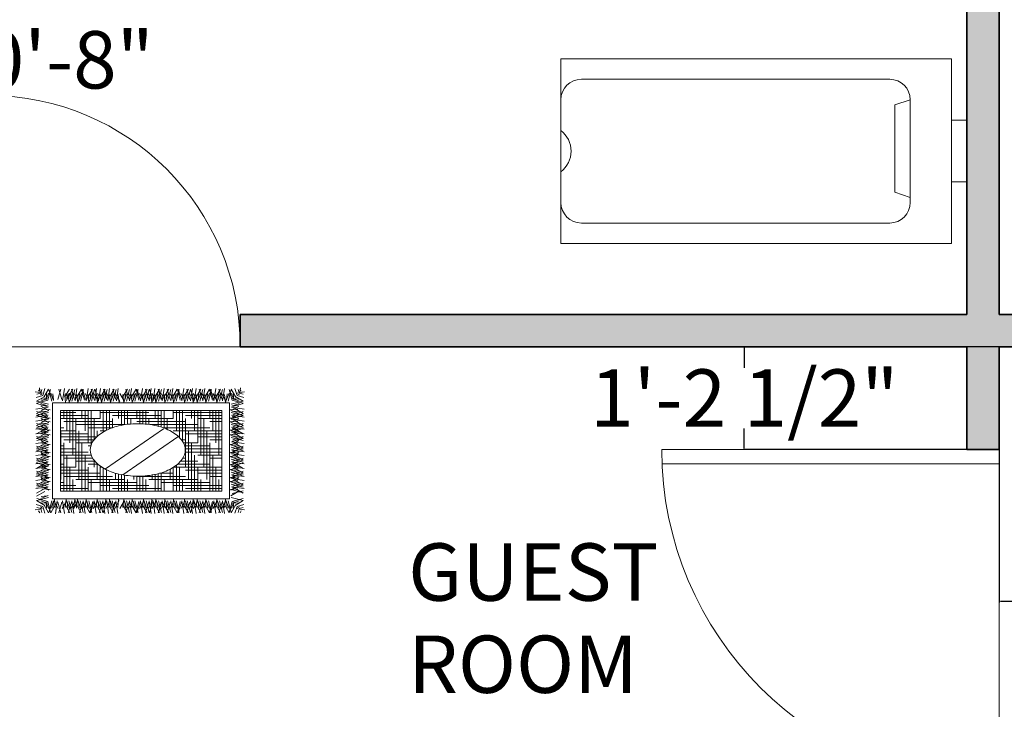
# Model space of a CAD drawing. Units: inches. Extents: x 638 to 1303, y 1 to 699.
# Tile 3 of 21: x 718 to 855, y 156 to 252. Entities that reach past the tile are written whole.
import ezdxf

# ---------------------------------------------------------------- set-up
doc = ezdxf.new("R2010")
doc.units = ezdxf.units.IN
doc.header["$MEASUREMENT"] = 0
for name, color, linetype, lineweight in [('A-ANNO-DIMS', 2, 'Continuous', 18), ('A-AREA-IDEN', 7, 'Continuous', 18), ('A-DOOR', 4, 'Continuous', 18), ('A-FLOR-FIXT', 9, 'Continuous', 18), ('A-FURN-PATT', 8, 'Continuous', 13), ('A-FURN-RUGS', 8, 'Continuous', 13), ('A-WALL', 7, 'Continuous', 35)]:
    doc.layers.add(name, color=color, linetype=linetype, lineweight=lineweight)
doc.layers.add('A-WALL-PATT', color=143, linetype='Continuous', lineweight=13, true_color=0x7aafdf)
doc.styles.get("Standard").update_dxf_attribs({"font": 'arial.ttf'})
doc.dimstyles.get("Standard").update_dxf_attribs({"dimtxt": 8, "dimasz": 0.18, "dimexe": 0.18, "dimexo": 0.0625, "dimgap": 0.09, "dimtad": 0, "dimtih": 1, "dimtoh": 1, "dimdec": 4, "dimzin": 0, "dimdsep": 46, "dimlunit": 3, "dimtxsty": 'Standard', "dimcen": 0.09, "dimadec": 0, "dimazin": 0, "dimtfac": 1, "dimtdec": 4, "dimtofl": 0, "dimtmove": 0, "dimatfit": 3, "dimfxl": 1, "dimtolj": 1, "dimtzin": 0, "dimarcsym": 0})

# ---------------------------------------------------------------- blocks, each defined once
blk = doc.blocks.new('DOOR-SWING-47')
for p, q in [((45, 0), (45, 46.96)), ((47, 0), (47, 47)), ((0, 0), (47, 0))]:
    blk.add_line(p, q)
blk.add_arc((47, 0), 47, 90, 180)
blk = doc.blocks.new('DOOR-SWING-35')
for p, q in [((33, 0), (33, 34.94)), ((35, 0), (35, 35)), ((0, 0), (35, 0))]:
    blk.add_line(p, q)
blk.add_arc((35, 0), 35, 90, 180)
blk = doc.blocks.new('*D30')
at = {"layer": 'A-ANNO-DIMS', "color": 0, "lineweight": -2, "transparency": 16777216}
for p, q in [((913.6, 276.19), (909.79, 276.19)), ((909.97, 276.01), (909.97, 268.11)), ((909.97, 251.76), (909.97, 259.66)), ((913.6, 251.58), (909.79, 251.58))]:
    blk.add_line(p, q, dxfattribs=at)
at = {"layer": 'A-ANNO-DIMS', "color": 0, "transparency": 16777216}
for points in [[(909.94, 276.01), (910, 276.01), (909.97, 276.19)], [(909.94, 251.76), (910, 251.76), (909.97, 251.58)]]:
    blk.add_solid(points, dxfattribs=at)
at = {"layer": 'Defpoints', "color": 0, "transparency": 16777216}
for p in [(913.67, 276.19), (909.97, 251.58), (913.67, 251.58)]:
    blk.add_point(p, dxfattribs=at)
at = {"layer": 'A-ANNO-DIMS', "color": 0, "transparency": 16777216, "insert": (909.97, 263.89), "char_height": 8, "attachment_point": 5}
blk.add_mtext('\\A1;DINING CHAIR 2\'-0 1/2" TYP.', dxfattribs=at)
blk = doc.blocks.new('*D61')
at = {"layer": 'A-ANNO-DIMS', "color": 0, "lineweight": -2, "transparency": 16777216}
for p, q in [((854.74, 206.76), (854.74, 171.14)), ((923.85, 206.76), (923.85, 171.14)), ((854.92, 171.32), (878.57, 171.32)), ((923.67, 171.32), (900.02, 171.32))]:
    blk.add_line(p, q, dxfattribs=at)
at = {"layer": 'A-ANNO-DIMS', "color": 0, "transparency": 16777216}
for points in [[(854.92, 171.35), (854.92, 171.29), (854.74, 171.32)], [(923.67, 171.35), (923.67, 171.29), (923.85, 171.32)]]:
    blk.add_solid(points, dxfattribs=at)
at = {"layer": 'Defpoints', "color": 0, "transparency": 16777216}
for p in [(854.74, 206.82), (923.85, 206.82), (854.74, 171.32)]:
    blk.add_point(p, dxfattribs=at)
at = {"layer": 'A-ANNO-DIMS', "color": 0, "transparency": 16777216, "insert": (889.29, 171.32), "char_height": 8, "attachment_point": 5}
blk.add_mtext('\\A1;5\'-9"', dxfattribs=at)
blk = doc.blocks.new('*D63')
at = {"layer": 'A-ANNO-DIMS', "color": 0, "lineweight": -2, "transparency": 16777216}
for p, q in [((854.68, 206.82), (819.06, 206.82)), ((819.24, 206.64), (819.24, 203.89)), ((819.24, 192.68), (819.24, 195.43)), ((854.68, 192.5), (819.06, 192.5))]:
    blk.add_line(p, q, dxfattribs=at)
at = {"layer": 'A-ANNO-DIMS', "color": 0, "transparency": 16777216}
for points in [[(819.21, 206.64), (819.27, 206.64), (819.24, 206.82)], [(819.21, 192.68), (819.27, 192.68), (819.24, 192.5)]]:
    blk.add_solid(points, dxfattribs=at)
at = {"layer": 'Defpoints', "color": 0, "transparency": 16777216}
for p in [(819.24, 206.82), (854.74, 206.82), (854.74, 192.5)]:
    blk.add_point(p, dxfattribs=at)
at = {"layer": 'A-ANNO-DIMS', "color": 0, "transparency": 16777216, "insert": (819.24, 199.66), "char_height": 8, "attachment_point": 5}
blk.add_mtext('\\A1;1\'-2 1/2"', dxfattribs=at)
blk = doc.blocks.new('*D71')
at = {"layer": 'A-ANNO-DIMS', "color": 0, "lineweight": -2, "transparency": 16777216}
for p, q in [((706.24, 211.38), (706.24, 247)), ((714.01, 211.38), (714.01, 247)), ((706.42, 246.82), (713.83, 246.82)), ((714.01, 246.82), (714.19, 246.82))]:
    blk.add_line(p, q, dxfattribs=at)
at = {"layer": 'A-ANNO-DIMS', "color": 0, "transparency": 16777216}
for points in [[(706.42, 246.85), (706.42, 246.79), (706.24, 246.82)], [(713.83, 246.85), (713.83, 246.79), (714.01, 246.82)]]:
    blk.add_solid(points, dxfattribs=at)
at = {"layer": 'Defpoints', "color": 0, "transparency": 16777216}
for p in [(714.01, 246.82), (706.24, 211.32), (714.01, 211.32)]:
    blk.add_point(p, dxfattribs=at)
at = {"layer": 'A-ANNO-DIMS', "color": 0, "transparency": 16777216, "insert": (724.91, 246.82), "char_height": 8, "attachment_point": 5}
blk.add_mtext('\\A1;0\'-8"', dxfattribs=at)

msp = doc.modelspace()

# ---------------------------------------------------------------- hatches: boundary and pattern name
at = {"layer": 'A-FURN-PATT'}
h = msp.add_hatch(dxfattribs=at)
h.set_pattern_fill('HOUND', color=256, scale=6.7861, angle=90, style=0)
h.paths.add_polyline_path([(746.43034, 197.90061), (723.94396, 197.90061), (723.94396, 186.67691), (746.43034, 186.67691)])
h.paths.add_polyline_path([(728.47502, 191.24073), (728.41875, 191.32863), (728.3669, 191.4192), (728.3196, 191.51224), (728.27696, 191.60749), (728.23909, 191.70475), (728.20608, 191.80375), (728.178, 191.90427), (728.15494, 192.00606), (728.13695, 192.10886), (728.12406, 192.21243), (728.11632, 192.31651), (728.11373, 192.42084), (728.11632, 192.52518), (728.12406, 192.62926), (728.13695, 192.73282), (728.15494, 192.83563), (728.178, 192.93741), (728.20608, 193.03793), (728.23909, 193.13694), (728.27696, 193.23419), (728.3196, 193.32945), (728.3669, 193.42248), (728.41875, 193.51306), (728.47502, 193.60096), (728.53557, 193.68596), (728.67485, 193.86279), (728.82227, 194.03288), (728.97752, 194.19587), (729.14025, 194.35138), (729.3101, 194.49909), (729.4867, 194.63866), (729.66966, 194.76978), (729.85857, 194.89217), (730.05301, 195.00555), (730.37297, 195.17259), (730.70035, 195.32453), (731.03447, 195.46106), (731.37457, 195.58187), (731.71994, 195.68671), (732.06982, 195.77534), (732.59633, 195.88335), (733.12717, 195.96758), (733.66125, 196.02787), (734.19751, 196.06409), (734.73485, 196.07618), (735.27219, 196.06409), (735.80845, 196.02787), (736.34253, 195.96758), (736.87337, 195.88335), (737.39988, 195.77534), (737.74976, 195.68671), (738.09513, 195.58187), (738.43523, 195.46106), (738.76935, 195.32453), (739.09673, 195.17259), (739.41669, 195.00555), (739.61113, 194.89217), (739.80004, 194.76978), (739.983, 194.63866), (740.1596, 194.49909), (740.32945, 194.35138), (740.49218, 194.19587), (740.64743, 194.03288), (740.79485, 193.86279), (740.93413, 193.68596), (740.99468, 193.60096), (741.05095, 193.51306), (741.1028, 193.42248), (741.1501, 193.32945), (741.19274, 193.23419), (741.23061, 193.13694), (741.26362, 193.03793), (741.29169, 192.93741), (741.31476, 192.83563), (741.33275, 192.73282), (741.34564, 192.62926), (741.35338, 192.52518), (741.35597, 192.42084), (741.35338, 192.31651), (741.34564, 192.21243), (741.33275, 192.10886), (741.31476, 192.00606), (741.29169, 191.90427), (741.26362, 191.80375), (741.23061, 191.70475), (741.19274, 191.60749), (741.1501, 191.51224), (741.1028, 191.4192), (741.05095, 191.32863), (740.99468, 191.24073), (740.93413, 191.15572), (740.79485, 190.9789), (740.64743, 190.8088), (740.49218, 190.64582), (740.32945, 190.4903), (740.1596, 190.3426), (739.983, 190.20303), (739.80004, 190.07191), (739.61113, 189.94952), (739.41669, 189.83613), (739.09673, 189.6691), (738.76935, 189.51716), (738.43523, 189.38063), (738.09513, 189.25981), (737.74976, 189.15498), (737.39988, 189.06634), (736.87337, 188.95833), (736.34253, 188.8741), (735.80845, 188.81381), (735.27219, 188.77759), (734.73485, 188.76551), (734.19751, 188.77759), (733.66125, 188.81381), (733.12717, 188.8741), (732.59633, 188.95833), (732.06982, 189.06634), (731.71994, 189.15498), (731.37457, 189.25981), (731.03447, 189.38063), (730.70035, 189.51716), (730.37297, 189.6691), (730.05301, 189.83613), (729.85857, 189.94952), (729.66966, 190.07191), (729.4867, 190.20303), (729.3101, 190.3426), (729.14025, 190.4903), (728.97752, 190.64582), (728.82227, 190.8088), (728.67485, 190.9789), (728.53557, 191.15572)], flags=0)
at = {"layer": 'A-WALL-PATT'}
h = msp.add_hatch(color=256, dxfattribs=at)
h.dxf.hatch_style = 1
h.paths.add_polyline_path([(973.34524, 629.81895), (793.35541, 629.81895), (793.35541, 620.81895), (850.23798, 620.81895), (922.23798, 620.81895), (922.23798, 524.81895), (908.94335, 524.81895), (908.94335, 520.31895), (926.73798, 520.31895), (926.73798, 544.31895), (979.3571, 544.31895), (979.3571, 548.81895), (926.73798, 548.81895), (926.73798, 620.81895), (973.34524, 620.81895)])
h.paths.add_polyline_path([(758.35541, 629.81895), (697.23798, 629.81895), (697.23798, 586.77451), (706.23798, 586.77451), (706.23798, 620.81895), (758.35541, 620.81895)])
h.paths.add_polyline_path([(1075.85281, 629.81895), (1003.34524, 629.81895), (1003.34524, 620.81895), (1046.73798, 620.81895), (1046.73798, 560.81895), (1046.73798, 548.81895), (1026.3571, 548.81895), (1026.3571, 544.31895), (1046.73798, 544.31895), (1046.73798, 486.87457), (1051.23798, 486.87457), (1051.23798, 556.31895), (1162.89753, 556.31895), (1162.89753, 560.81895), (1051.23798, 560.81895), (1051.23798, 620.81895), (1075.85281, 620.81895)])
h.paths.add_polyline_path([(1228.23798, 629.81895), (1105.85281, 629.81895), (1105.85281, 620.81895), (1219.23798, 620.81895), (1219.23798, 560.81895), (1197.89753, 560.81895), (1197.89753, 556.31895), (1219.23798, 556.31895), (1219.23798, 498.80084), (1228.23798, 498.80084)])
h.paths.add_polyline_path([(1051.23798, 439.87457), (1046.73798, 439.87457), (1046.73798, 407.81895), (1219.23798, 407.81895), (1219.23798, 381.66175), (1228.23798, 381.66175), (1228.23798, 451.80084), (1219.23798, 451.80084), (1219.23798, 412.31895), (1051.23798, 412.31895)])
h.paths.add_polyline_path([(1228.23798, 346.66175), (1219.23798, 346.66175), (1219.23798, 335.81895), (1046.73798, 335.81895), (1046.73798, 273.56895), (1051.23798, 273.56895), (1051.23798, 331.31895), (1219.23798, 331.31895), (1219.23798, 308.99654), (1228.23798, 308.99654)])
h.paths.add_polyline_path([(1228.23798, 261.99654), (1219.23798, 261.99654), (1219.23798, 211.31895), (1051.23798, 211.31895), (1051.23798, 226.56895), (1046.73798, 226.56895), (1046.73798, 211.31895), (983.84714, 211.31895), (983.84714, 206.81895), (1219.23798, 206.81895), (1219.23798, 166.83987), (1228.23798, 166.83987)])
h.paths.add_polyline_path([(1228.23798, 119.83987), (1219.23798, 119.83987), (1219.23798, 50.81895), (1197.89277, 50.81895), (1197.89277, 41.81895), (1228.23798, 41.81895)])
h.paths.add_polyline_path([(1162.89277, 50.81895), (1069.02949, 50.81895), (1069.02949, 41.81895), (1162.89277, 41.81895)])
h.paths.add_polyline_path([(1010.02949, 50.81895), (941.89631, 50.81895), (917.77455, 50.81895), (917.77455, 41.81895), (941.89631, 41.81895), (1010.02949, 41.81895)])
h.paths.add_polyline_path([(882.77455, 50.81895), (854.73798, 50.81895), (854.73798, 145.50379), (850.23798, 145.50379), (850.23798, 50.81895), (793.49755, 50.81895), (793.49755, 41.81895), (882.77455, 41.81895)])
h.paths.add_polyline_path([(746.49755, 50.81895), (706.23798, 50.81895), (706.23798, 96.57416), (697.23798, 96.57416), (697.23798, 41.81895), (746.49755, 41.81895)])
h.paths.add_polyline_path([(706.23798, 206.81895), (714.01165, 206.81895), (714.01165, 211.31895), (706.23798, 211.31895), (706.23798, 251.21966), (697.23798, 251.21966), (697.23798, 143.57416), (706.23798, 143.57416)])
h.paths.add_polyline_path([(923.84714, 211.31895), (854.73798, 211.31895), (854.73798, 397.8313), (850.23798, 397.8313), (850.23798, 388.31895), (747.9539, 388.31895), (747.9539, 383.81895), (850.23798, 383.81895), (850.23798, 311.81895), (706.23798, 311.81895), (706.23798, 342.78787), (697.23798, 342.78787), (697.23798, 281.21966), (706.23798, 281.21966), (706.23798, 307.31895), (850.23798, 307.31895), (850.23798, 211.31895), (749.01165, 211.31895), (749.01165, 206.81895), (850.23798, 206.81895), (850.23798, 192.50379), (854.73798, 192.50379), (854.73798, 206.81895), (923.84714, 206.81895)])
h.paths.add_polyline_path([(706.23798, 434.70471), (697.23798, 434.70471), (697.23798, 372.78787), (706.23798, 372.78787), (706.23798, 383.81895), (712.9539, 383.81895), (712.9539, 388.31895), (706.23798, 388.31895)])
h.paths.add_polyline_path([(706.23798, 520.31895), (850.23798, 520.31895), (850.23798, 444.8313), (854.73798, 444.8313), (854.73798, 520.31895), (861.94335, 520.31895), (861.94335, 524.81895), (706.23798, 524.81895), (706.23798, 551.77451), (697.23798, 551.77451), (697.23798, 481.70471), (706.23798, 481.70471)])

# ---------------------------------------------------------------- linework, layer by layer
at = {"layer": 'A-FLOR-FIXT'}
for p, q in [((848.09005, 246.97327), (793.67582, 246.97327)), ((793.67582, 246.97327), (793.67582, 221.19811)), ((848.09005, 221.19811), (848.09005, 246.97327)), ((839.49833, 244.10937), (796.53973, 244.10937)), ((842.36224, 241.24546), (840.21431, 240.52948)), ((840.21431, 228.35788), (840.21431, 240.52948)), ((842.36224, 226.92593), (842.36224, 241.24546)), ((848.09005, 238.38155), (850.23798, 238.38155)), ((850.23798, 238.38155), (850.23798, 229.78983)), ((848.09005, 229.78983), (850.23798, 229.78983)), ((842.36224, 227.6419), (840.21431, 228.35788)), ((796.53973, 224.06202), (839.49833, 224.06202)), ((793.67582, 221.19811), (848.09005, 221.19811))]:
    msp.add_line(p, q, dxfattribs=at)
for centre, radius, start, end in [((796.53973, 241.24546), 2.86391, 90, 180), ((839.49833, 241.24546), 2.86391, 0, 90), ((791.52789, 234.08569), 3.57988, 306.869898, 53.130102), ((796.53973, 226.92593), 2.86391, 180, 270), ((839.49833, 226.92593), 2.86391, 270, 0)]:
    msp.add_arc(centre, radius, start, end, dxfattribs=at)
at = {"layer": 'A-FURN-RUGS'}
for p, q in [((721.11872, 200.41749), (720.45866, 200.51713)), ((721.21475, 200.32147), (720.67085, 200.17846)), ((720.9151, 200.62111), (721.07888, 200.9029)), ((721.11872, 200.41749), (721.01909, 201.07755)), ((721.21475, 200.32147), (721.35775, 200.86537)), ((721.33547, 200.20074), (721.43162, 200.37259)), ((721.50616, 200.03006), (721.79097, 200.97367)), ((721.65306, 199.76082), (722.31683, 200.9029)), ((721.99987, 199.53634), (722.3001, 200.33103)), ((722.19497, 199.34124), (722.5957, 200.86537)), ((722.75262, 199.23847), (722.32488, 200.86537)), ((723.01132, 199.2965), (722.62048, 200.33103)), ((723.58084, 199.44967), (724.02005, 200.90476)), ((724.17121, 199.44967), (723.732, 200.90476)), ((724.24114, 199.26803), (724.50389, 201.00865)), ((724.53462, 199.76082), (725.19839, 200.9029)), ((725.27502, 199.1818), (724.64727, 200.30368)), ((724.79082, 199.2965), (725.18166, 200.33103)), ((725.04045, 199.76082), (725.70422, 200.9029)), ((725.29665, 199.2965), (725.68749, 200.33103)), ((725.93028, 199.44967), (725.49108, 200.90476)), ((725.55534, 199.23847), (725.98309, 200.86537)), ((726.47818, 199.1818), (725.85043, 200.30368)), ((726.00022, 199.26803), (726.26297, 201.00865)), ((726.24361, 199.76082), (726.90738, 200.9029)), ((726.49981, 199.2965), (726.89065, 200.33103)), ((726.7585, 199.23847), (727.18625, 200.86537)), ((727.31615, 199.34124), (726.91542, 200.86537)), ((727.46765, 199.44967), (727.02845, 200.90476)), ((728.01555, 199.1818), (727.3878, 200.30368)), ((727.53759, 199.26803), (727.80034, 201.00865)), ((727.78098, 199.76082), (728.44475, 200.9029)), ((728.03718, 199.2965), (728.42802, 200.33103)), ((728.67082, 199.44967), (728.23161, 200.90476)), ((728.29587, 199.23847), (728.72362, 200.86537)), ((729.21871, 199.1818), (728.59096, 200.30368)), ((728.74075, 199.26803), (729.0035, 201.00865)), ((729.20555, 199.44967), (728.76635, 200.90476)), ((729.75345, 199.1818), (729.1257, 200.30368)), ((729.27549, 199.26803), (729.53824, 201.00865)), ((729.51888, 199.76082), (730.18265, 200.9029)), ((729.77508, 199.2965), (730.16592, 200.33103)), ((730.40872, 199.44967), (729.96951, 200.90476)), ((730.03377, 199.23847), (730.46152, 200.86537)), ((730.47556, 199.44967), (730.03635, 200.90476)), ((731.02345, 199.1818), (730.3957, 200.30368)), ((730.54549, 199.26803), (730.80824, 201.00865)), ((730.78888, 199.76082), (731.45265, 200.9029)), ((731.04508, 199.2965), (731.43592, 200.33103)), ((731.67872, 199.44967), (731.23951, 200.90476)), ((731.30377, 199.23847), (731.73152, 200.86537)), ((732.22662, 199.1818), (731.59886, 200.30368)), ((731.74865, 199.26803), (732.0114, 201.00865)), ((732.86243, 199.1818), (732.23468, 200.30368)), ((732.62786, 199.76082), (733.29162, 200.9029)), ((732.88406, 199.2965), (733.27489, 200.33103)), ((733.51769, 199.44967), (733.07849, 200.90476)), ((733.14275, 199.23847), (733.57049, 200.86537)), ((734.06559, 199.1818), (733.43784, 200.30368)), ((733.58763, 199.26803), (733.85037, 201.00865)), ((733.83102, 199.76082), (734.49479, 200.9029)), ((734.08722, 199.2965), (734.47805, 200.33103)), ((734.34591, 199.23847), (734.77366, 200.86537)), ((734.90356, 199.34124), (734.50283, 200.86537)), ((735.05506, 199.44967), (734.61586, 200.90476)), ((735.60296, 199.1818), (734.97521, 200.30368)), ((735.125, 199.26803), (735.38775, 201.00865)), ((735.36839, 199.76082), (736.03216, 200.9029)), ((735.62459, 199.2965), (736.01543, 200.33103)), ((736.25822, 199.44967), (735.81902, 200.90476)), ((735.88328, 199.23847), (736.31103, 200.86537)), ((736.80612, 199.1818), (736.17837, 200.30368)), ((736.32816, 199.26803), (736.59091, 201.00865)), ((736.79296, 199.44967), (736.35376, 200.90476)), ((737.34086, 199.1818), (736.71311, 200.30368)), ((736.8629, 199.26803), (737.12565, 201.00865)), ((737.10629, 199.76082), (737.77006, 200.9029)), ((737.36249, 199.2965), (737.75333, 200.33103)), ((737.99612, 199.44967), (737.55692, 200.90476)), ((737.62118, 199.23847), (738.04893, 200.86537)), ((738.06296, 199.44967), (737.62376, 200.90476)), ((738.61086, 199.1818), (737.98311, 200.30368)), ((738.1329, 199.26803), (738.39565, 201.00865)), ((738.37629, 199.76082), (739.04006, 200.9029)), ((738.63249, 199.2965), (739.02333, 200.33103)), ((739.26612, 199.44967), (738.82692, 200.90476)), ((738.89118, 199.23847), (739.31893, 200.86537)), ((739.81402, 199.1818), (739.18627, 200.30368)), ((739.33606, 199.26803), (739.59881, 201.00865)), ((739.57945, 199.76082), (740.24322, 200.9029)), ((739.83565, 199.2965), (740.22649, 200.33103)), ((740.09434, 199.23847), (740.52209, 200.86537)), ((740.65199, 199.34124), (740.25127, 200.86537)), ((740.8035, 199.44967), (740.36429, 200.90476)), ((741.3514, 199.1818), (740.72365, 200.30368)), ((740.87343, 199.26803), (741.13618, 201.00865)), ((741.11682, 199.76082), (741.78059, 200.9029)), ((741.37303, 199.2965), (741.76386, 200.33103)), ((742.00666, 199.44967), (741.56746, 200.90476)), ((741.63172, 199.23847), (742.05946, 200.86537)), ((742.55456, 199.1818), (741.92681, 200.30368)), ((742.0766, 199.26803), (742.33934, 201.00865)), ((742.5414, 199.44967), (742.10219, 200.90476)), ((743.0893, 199.1818), (742.46155, 200.30368)), ((742.61133, 199.26803), (742.87408, 201.00865)), ((742.85473, 199.76082), (743.51849, 200.9029)), ((743.11093, 199.2965), (743.50176, 200.33103)), ((743.74456, 199.44967), (743.30536, 200.90476)), ((743.36962, 199.23847), (743.79736, 200.86537)), ((744.29246, 199.1818), (743.66471, 200.30368)), ((743.8145, 199.26803), (744.07724, 201.00865)), ((744.05789, 199.76082), (744.72166, 200.9029)), ((744.31409, 199.2965), (744.70492, 200.33103)), ((744.57278, 199.23847), (745.00053, 200.86537)), ((745.13043, 199.34124), (744.7297, 200.86537)), ((745.28193, 199.44967), (744.84273, 200.90476)), ((745.82983, 199.1818), (745.20208, 200.30368)), ((745.35187, 199.26803), (745.61462, 201.00865)), ((745.59526, 199.76082), (746.25903, 200.9029)), ((745.85146, 199.2965), (746.2423, 200.33103)), ((746.48509, 199.44967), (746.04589, 200.90476)), ((746.11015, 199.23847), (746.5379, 200.86537)), ((747.03299, 199.1818), (746.40524, 200.30368)), ((746.55503, 199.26803), (746.81778, 201.00865)), ((747.05462, 199.2965), (747.44546, 200.33103)), ((747.31331, 199.23847), (747.74106, 200.86537)), ((747.87096, 199.34124), (747.47023, 200.86537)), ((748.41287, 199.76082), (747.74911, 200.9029)), ((748.06606, 199.53634), (747.76584, 200.33103)), ((748.55978, 200.03006), (748.27496, 200.97367)), ((748.73047, 200.20074), (748.63431, 200.37259)), ((748.85119, 200.32147), (748.70819, 200.86537)), ((748.85119, 200.32147), (749.39509, 200.17846)), ((748.94721, 200.41749), (749.04685, 201.07755)), ((748.94721, 200.41749), (749.60727, 200.51713)), ((749.15083, 200.62111), (748.98706, 200.9029)), ((721.50616, 200.03006), (720.56255, 199.74524)), ((721.77539, 199.88315), (720.63332, 199.21938)), ((722.19497, 199.34124), (720.67085, 198.94051)), ((722.29774, 198.78359), (720.67085, 199.21134)), ((722.29774, 198.78359), (720.67085, 199.21134)), ((721.33547, 200.20074), (721.16363, 200.10459)), ((721.99987, 199.53634), (721.20519, 199.23611)), ((722.23971, 198.5249), (721.20519, 198.91573)), ((722.23971, 198.5249), (721.20519, 198.91573)), ((722.13213, 199.58515), (721.27812, 199.5053)), ((721.95106, 199.40409), (722.03091, 200.2581)), ((747.51611, 198.98639), (722.85818, 198.98639)), ((722.85818, 198.98639), (722.85818, 185.59114)), ((722.96952, 199.40409), (722.88967, 200.2581)), ((724.67498, 199.00804), (724.55557, 200.16633)), ((724.83262, 199.40409), (724.91247, 200.2581)), ((725.1808, 199.00804), (725.0614, 200.16633)), ((725.33845, 199.40409), (725.4183, 200.2581)), ((726.38396, 199.00804), (726.26456, 200.16633)), ((726.54161, 199.40409), (726.62146, 200.2581)), ((727.92134, 199.00804), (727.80193, 200.16633)), ((728.07898, 199.40409), (728.15883, 200.2581)), ((729.1245, 199.00804), (729.00509, 200.16633)), ((729.65924, 199.00804), (729.53983, 200.16633)), ((729.81688, 199.40409), (729.89673, 200.2581)), ((730.92924, 199.00804), (730.80983, 200.16633)), ((731.08688, 199.40409), (731.16673, 200.2581)), ((732.1324, 199.00804), (732.01299, 200.16633)), ((732.76821, 199.00804), (732.6488, 200.16633)), ((732.92585, 199.40409), (733.00571, 200.2581)), ((733.97137, 199.00804), (733.85196, 200.16633)), ((734.12901, 199.40409), (734.20887, 200.2581)), ((735.50874, 199.00804), (735.38934, 200.16633)), ((735.66639, 199.40409), (735.74624, 200.2581)), ((736.71191, 199.00804), (736.5925, 200.16633)), ((737.24664, 199.00804), (737.12724, 200.16633)), ((737.40429, 199.40409), (737.48414, 200.2581)), ((738.51665, 199.00804), (738.39724, 200.16633)), ((738.67429, 199.40409), (738.75414, 200.2581)), ((739.71981, 199.00804), (739.6004, 200.16633)), ((739.87745, 199.40409), (739.9573, 200.2581)), ((741.25718, 199.00804), (741.13777, 200.16633)), ((741.41482, 199.40409), (741.49468, 200.2581)), ((742.46034, 199.00804), (742.34093, 200.16633)), ((742.99508, 199.00804), (742.87567, 200.16633)), ((743.15272, 199.40409), (743.23258, 200.2581)), ((744.19824, 199.00804), (744.07883, 200.16633)), ((744.35588, 199.40409), (744.43574, 200.2581)), ((745.73561, 199.00804), (745.61621, 200.16633)), ((745.89326, 199.40409), (745.97311, 200.2581)), ((746.93878, 199.00804), (746.81937, 200.16633)), ((747.09642, 199.40409), (747.17627, 200.2581)), ((747.09642, 199.40409), (747.17627, 200.2581)), ((747.51611, 185.59114), (747.51611, 198.98639)), ((747.76819, 198.78359), (749.39509, 199.21134)), ((747.76819, 198.78359), (749.39509, 199.21134)), ((747.82622, 198.5249), (748.86075, 198.91573)), ((747.82622, 198.5249), (748.86075, 198.91573)), ((747.87096, 199.34124), (749.39509, 198.94051)), ((747.93381, 199.58515), (748.78782, 199.5053)), ((748.11488, 199.40409), (748.03502, 200.2581)), ((748.06606, 199.53634), (748.86075, 199.23611)), ((748.29054, 199.88315), (749.43262, 199.21938)), ((748.55978, 200.03006), (749.50339, 199.74524)), ((748.73047, 200.20074), (748.90231, 200.10459)), ((722.26818, 198.39236), (720.52757, 198.12961)), ((722.08654, 198.46229), (720.63145, 198.9015)), ((722.08654, 197.32517), (720.63145, 197.76437)), ((721.77539, 198.14897), (720.63332, 197.4852)), ((721.77539, 198.14897), (720.63332, 197.4852)), ((722.29774, 197.63407), (720.67085, 197.20633)), ((722.29774, 197.63407), (720.67085, 197.20633)), ((722.23971, 197.89276), (721.20519, 197.50193)), ((722.23971, 197.89276), (721.20519, 197.50193)), ((722.35441, 197.91439), (721.23253, 198.54214)), ((722.13213, 198.56669), (721.27812, 198.64655)), ((722.13213, 198.56669), (721.27812, 198.64655)), ((722.13213, 197.85097), (721.27812, 197.77111)), ((722.13213, 197.85097), (721.27812, 197.77111)), ((722.52817, 198.00861), (721.36988, 198.12802)), ((746.43034, 197.90061), (723.94396, 197.90061)), ((723.94396, 197.90061), (723.94396, 186.67691)), ((746.43034, 186.67691), (746.43034, 197.90061)), ((747.53777, 198.00861), (748.69605, 198.12802)), ((747.71153, 197.91439), (748.83341, 198.54214)), ((747.76819, 197.63407), (749.39509, 197.20633)), ((747.76819, 197.63407), (749.39509, 197.20633)), ((747.79775, 198.39236), (749.53837, 198.12961)), ((747.82622, 197.89276), (748.86075, 197.50193)), ((747.82622, 197.89276), (748.86075, 197.50193)), ((747.93381, 198.56669), (748.78782, 198.64655)), ((747.93381, 198.56669), (748.78782, 198.64655)), ((747.93381, 197.85097), (748.78782, 197.77111)), ((747.93381, 197.85097), (748.78782, 197.77111)), ((747.9794, 198.46229), (749.43449, 198.9015)), ((747.9794, 197.32517), (749.43449, 197.76437)), ((748.29054, 198.14897), (749.43262, 197.4852)), ((748.29054, 198.14897), (749.43262, 197.4852)), ((722.26818, 197.25523), (720.52757, 196.99248)), ((722.26818, 196.72012), (720.52757, 196.45737)), ((722.08654, 196.79005), (720.63145, 197.22926)), ((721.77539, 196.47672), (720.63332, 195.81296)), ((721.77539, 196.47672), (720.63332, 195.81296)), ((722.19497, 197.07642), (720.67085, 197.47715)), ((722.23971, 196.22052), (721.20519, 195.82969)), ((722.23971, 196.22052), (721.20519, 195.82969)), ((722.35441, 196.77727), (721.23253, 197.40502)), ((722.35441, 196.24215), (721.23253, 196.8699)), ((722.13213, 196.71384), (721.27812, 196.63399)), ((722.13213, 196.71384), (721.27812, 196.63399)), ((722.13213, 196.17873), (721.27812, 196.09887)), ((722.13213, 196.17873), (721.27812, 196.09887)), ((722.52817, 196.87148), (721.36988, 196.99089)), ((722.52817, 196.33637), (721.36988, 196.45578)), ((747.53777, 196.87148), (748.69605, 196.99089)), ((747.53777, 196.33637), (748.69605, 196.45578)), ((747.71153, 196.77727), (748.83341, 197.40502)), ((747.71153, 196.24215), (748.83341, 196.8699)), ((747.79775, 197.25523), (749.53837, 196.99248)), ((747.79775, 196.72012), (749.53837, 196.45737)), ((747.82622, 196.22052), (748.86075, 195.82969)), ((747.82622, 196.22052), (748.86075, 195.82969)), ((747.87096, 197.07642), (749.39509, 197.47715)), ((747.93381, 196.71384), (748.78782, 196.63399)), ((747.93381, 196.71384), (748.78782, 196.63399)), ((747.93381, 196.17873), (748.78782, 196.09887)), ((747.93381, 196.17873), (748.78782, 196.09887)), ((747.9794, 196.79005), (749.43449, 197.22926)), ((748.29054, 196.47672), (749.43262, 195.81296)), ((748.29054, 196.47672), (749.43262, 195.81296)), ((722.26818, 195.58299), (720.52757, 195.32024)), ((722.26818, 194.91409), (720.52757, 194.65134)), ((722.08654, 195.65292), (720.63145, 196.09213)), ((722.08654, 194.98403), (720.63145, 195.42323)), ((721.77539, 195.3396), (720.63332, 194.67583)), ((721.77539, 195.3396), (720.63332, 194.67583)), ((722.29774, 195.96183), (720.67085, 195.53409)), ((722.29774, 195.96183), (720.67085, 195.53409)), ((722.19497, 195.40418), (720.67085, 195.80491)), ((722.23971, 195.0834), (721.20519, 194.69256)), ((722.23971, 195.0834), (721.20519, 194.69256)), ((722.35441, 195.10503), (721.23253, 195.73278)), ((722.35441, 194.43613), (721.23253, 195.06388)), ((722.13213, 195.0416), (721.27812, 194.96175)), ((722.13213, 195.0416), (721.27812, 194.96175)), ((722.52817, 195.19924), (721.36988, 195.31865)), ((730.25929, 189.78727), (738.31779, 195.34752)), ((747.53777, 195.19924), (748.69605, 195.31865)), ((747.71153, 195.10503), (748.83341, 195.73278)), ((747.71153, 194.43613), (748.83341, 195.06388)), ((747.76819, 195.96183), (749.39509, 195.53409)), ((747.76819, 195.96183), (749.39509, 195.53409)), ((747.79775, 195.58299), (749.53837, 195.32024)), ((747.79775, 194.91409), (749.53837, 194.65134)), ((747.82622, 195.0834), (748.86075, 194.69256)), ((747.82622, 195.0834), (748.86075, 194.69256)), ((747.87096, 195.40418), (749.39509, 195.80491)), ((747.93381, 195.0416), (748.78782, 194.96175)), ((747.93381, 195.0416), (748.78782, 194.96175)), ((747.9794, 195.65292), (749.43449, 196.09213)), ((747.9794, 194.98403), (749.43449, 195.42323)), ((748.29054, 195.3396), (749.43262, 194.67583)), ((748.29054, 195.3396), (749.43262, 194.67583)), ((722.26818, 193.57629), (720.52757, 193.31354)), ((722.08654, 193.8469), (720.63145, 194.2861)), ((722.08654, 193.64623), (720.63145, 194.08543)), ((721.77539, 194.6707), (720.63332, 194.00693)), ((721.77539, 194.6707), (720.63332, 194.00693)), ((722.29774, 194.15581), (720.67085, 193.72806)), ((722.29774, 194.15581), (720.67085, 193.72806)), ((722.19497, 193.59816), (720.67085, 193.99889)), ((722.23971, 194.4145), (721.20519, 194.02366)), ((722.23971, 194.4145), (721.20519, 194.02366)), ((722.35441, 193.09833), (721.23253, 193.72608)), ((722.13213, 194.3727), (721.27812, 194.29285)), ((722.13213, 194.3727), (721.27812, 194.29285)), ((722.52817, 194.53035), (721.36988, 194.64975)), ((732.66016, 188.94691), (740.32324, 194.23433)), ((747.53777, 194.53035), (748.69605, 194.64975)), ((747.71153, 193.09833), (748.83341, 193.72608)), ((747.76819, 194.15581), (749.39509, 193.72806)), ((747.76819, 194.15581), (749.39509, 193.72806)), ((747.79775, 193.57629), (749.53837, 193.31354)), ((747.82622, 194.4145), (748.86075, 194.02366)), ((747.82622, 194.4145), (748.86075, 194.02366)), ((747.87096, 193.59816), (749.39509, 193.99889)), ((747.93381, 194.3727), (748.78782, 194.29285)), ((747.93381, 194.3727), (748.78782, 194.29285)), ((747.9794, 193.8469), (749.43449, 194.2861)), ((747.9794, 193.64623), (749.43449, 194.08543)), ((748.29054, 194.6707), (749.43262, 194.00693)), ((748.29054, 194.6707), (749.43262, 194.00693)), ((722.26818, 192.43916), (720.52757, 192.17641)), ((722.08654, 192.5091), (720.63145, 192.9483)), ((722.08654, 191.97399), (720.63145, 192.41319)), ((721.77539, 193.3329), (720.63332, 192.66913)), ((721.77539, 193.3329), (720.63332, 192.66913)), ((722.29774, 192.81801), (720.67085, 192.39026)), ((722.29774, 192.81801), (720.67085, 192.39026)), ((722.19497, 192.26036), (720.67085, 192.66109)), ((722.23971, 193.0767), (721.20519, 192.68586)), ((722.23971, 193.0767), (721.20519, 192.68586)), ((722.35441, 191.9612), (721.23253, 192.58895)), ((722.13213, 193.0349), (721.27812, 192.95505)), ((722.13213, 193.0349), (721.27812, 192.95505)), ((722.52817, 193.19255), (721.36988, 193.31195)), ((722.52817, 192.05542), (721.36988, 192.17482)), ((747.53777, 193.19255), (748.69605, 193.31195)), ((747.53777, 192.05542), (748.69605, 192.17482)), ((747.71153, 191.9612), (748.83341, 192.58895)), ((747.76819, 192.81801), (749.39509, 192.39026)), ((747.76819, 192.81801), (749.39509, 192.39026)), ((747.79775, 192.43916), (749.53837, 192.17641)), ((747.82622, 193.0767), (748.86075, 192.68586)), ((747.82622, 193.0767), (748.86075, 192.68586)), ((747.87096, 192.26036), (749.39509, 192.66109)), ((747.93381, 193.0349), (748.78782, 192.95505)), ((747.93381, 193.0349), (748.78782, 192.95505)), ((747.9794, 192.5091), (749.43449, 192.9483)), ((747.9794, 191.97399), (749.43449, 192.41319)), ((748.29054, 193.3329), (749.43262, 192.66913)), ((748.29054, 193.3329), (749.43262, 192.66913)), ((722.26818, 191.90405), (720.52757, 191.6413)), ((722.26818, 190.76692), (720.52757, 190.50417)), ((722.08654, 190.83686), (720.63145, 191.27606)), ((721.77539, 191.66066), (720.63332, 190.99689)), ((721.77539, 191.66066), (720.63332, 190.99689)), ((722.29774, 191.14577), (720.67085, 190.71802)), ((722.29774, 191.14577), (720.67085, 190.71802)), ((722.19497, 190.58812), (720.67085, 190.98885)), ((722.23971, 191.40446), (721.20519, 191.01362)), ((722.23971, 191.40446), (721.20519, 191.01362)), ((722.35441, 191.42609), (721.23253, 192.05384)), ((722.35441, 190.28896), (721.23253, 190.91671)), ((722.13213, 191.89777), (721.27812, 191.81792)), ((722.13213, 191.89777), (721.27812, 191.81792)), ((722.13213, 191.36266), (721.27812, 191.28281)), ((722.13213, 191.36266), (721.27812, 191.28281)), ((722.52817, 191.5203), (721.36988, 191.63971)), ((747.53777, 191.5203), (748.69605, 191.63971)), ((747.71153, 191.42609), (748.83341, 192.05384)), ((747.71153, 190.28896), (748.83341, 190.91671)), ((747.76819, 191.14577), (749.39509, 190.71802)), ((747.76819, 191.14577), (749.39509, 190.71802)), ((747.79775, 191.90405), (749.53837, 191.6413)), ((747.79775, 190.76692), (749.53837, 190.50417)), ((747.82622, 191.40446), (748.86075, 191.01362)), ((747.82622, 191.40446), (748.86075, 191.01362)), ((747.87096, 190.58812), (749.39509, 190.98885)), ((747.93381, 191.89777), (748.78782, 191.81792)), ((747.93381, 191.89777), (748.78782, 191.81792)), ((747.93381, 191.36266), (748.78782, 191.28281)), ((747.93381, 191.36266), (748.78782, 191.28281)), ((747.9794, 190.83686), (749.43449, 191.27606)), ((748.29054, 191.66066), (749.43262, 190.99689)), ((748.29054, 191.66066), (749.43262, 190.99689)), ((722.26818, 190.09803), (720.52757, 189.83528)), ((722.08654, 190.16796), (720.63145, 190.60717)), ((722.08654, 189.03084), (720.63145, 189.47004)), ((721.77539, 190.52353), (720.63332, 189.85976)), ((721.77539, 190.52353), (720.63332, 189.85976)), ((721.77539, 189.85464), (720.63332, 189.19087)), ((721.77539, 189.85464), (720.63332, 189.19087)), ((722.29774, 189.33974), (720.67085, 188.912)), ((722.29774, 189.33974), (720.67085, 188.912)), ((722.23971, 190.26733), (721.20519, 189.87649)), ((722.23971, 190.26733), (721.20519, 189.87649)), ((722.23971, 189.59844), (721.20519, 189.2076)), ((722.23971, 189.59844), (721.20519, 189.2076)), ((722.35441, 189.62006), (721.23253, 190.24782)), ((722.13213, 190.22553), (721.27812, 190.14568)), ((722.13213, 190.22553), (721.27812, 190.14568)), ((722.13213, 189.55664), (721.27812, 189.47679)), ((722.13213, 189.55664), (721.27812, 189.47679)), ((722.52817, 190.38318), (721.36988, 190.50258)), ((722.52817, 189.71428), (721.36988, 189.83369)), ((747.53777, 190.38318), (748.69605, 190.50258)), ((747.53777, 189.71428), (748.69605, 189.83369)), ((747.71153, 189.62006), (748.83341, 190.24782)), ((747.76819, 189.33974), (749.39509, 188.912)), ((747.76819, 189.33974), (749.39509, 188.912)), ((747.79775, 190.09803), (749.53837, 189.83528)), ((747.82622, 190.26733), (748.86075, 189.87649)), ((747.82622, 190.26733), (748.86075, 189.87649)), ((747.82622, 189.59844), (748.86075, 189.2076)), ((747.82622, 189.59844), (748.86075, 189.2076)), ((747.93381, 190.22553), (748.78782, 190.14568)), ((747.93381, 190.22553), (748.78782, 190.14568)), ((747.93381, 189.55664), (748.78782, 189.47679)), ((747.93381, 189.55664), (748.78782, 189.47679)), ((747.9794, 190.16796), (749.43449, 190.60717)), ((747.9794, 189.03084), (749.43449, 189.47004)), ((748.29054, 190.52353), (749.43262, 189.85976)), ((748.29054, 190.52353), (749.43262, 189.85976)), ((748.29054, 189.85464), (749.43262, 189.19087)), ((748.29054, 189.85464), (749.43262, 189.19087)), ((722.26818, 188.9609), (720.52757, 188.69815)), ((722.26818, 188.42579), (720.52757, 188.16304)), ((722.08654, 188.49572), (720.63145, 188.93493)), ((721.77539, 188.1824), (720.63332, 187.51863)), ((721.77539, 188.1824), (720.63332, 187.51863)), ((722.19497, 188.78209), (720.67085, 189.18282)), ((722.35441, 188.48294), (721.23253, 189.11069)), ((722.35441, 187.94782), (721.23253, 188.57557)), ((722.13213, 188.41951), (721.27812, 188.33966)), ((722.13213, 188.41951), (721.27812, 188.33966)), ((722.52817, 188.57715), (721.36988, 188.69656)), ((722.52817, 188.04204), (721.36988, 188.16145)), ((747.53777, 188.57715), (748.69605, 188.69656)), ((747.53777, 188.04204), (748.69605, 188.16145)), ((747.71153, 188.48294), (748.83341, 189.11069)), ((747.71153, 187.94782), (748.83341, 188.57557)), ((747.79775, 188.9609), (749.53837, 188.69815)), ((747.79775, 188.42579), (749.53837, 188.16304)), ((747.87096, 188.78209), (749.39509, 189.18282)), ((747.93381, 188.41951), (748.78782, 188.33966)), ((747.93381, 188.41951), (748.78782, 188.33966)), ((747.9794, 188.49572), (749.43449, 188.93493)), ((748.29054, 188.1824), (749.43262, 187.51863)), ((748.29054, 188.1824), (749.43262, 187.51863)), ((722.26818, 187.28866), (720.52757, 187.02591)), ((722.08654, 187.3586), (720.63145, 187.7978)), ((721.77539, 187.04527), (720.63332, 186.3815)), ((721.77539, 187.04527), (720.63332, 186.3815)), ((721.77539, 186.64558), (720.63332, 185.98181)), ((721.77539, 186.64558), (720.63332, 185.98181)), ((722.29774, 187.6675), (720.67085, 187.23976)), ((722.29774, 187.6675), (720.67085, 187.23976)), ((722.19497, 187.10985), (720.67085, 187.51058)), ((722.23971, 187.9262), (721.20519, 187.53536)), ((722.23971, 187.9262), (721.20519, 187.53536)), ((722.35441, 186.8107), (721.23253, 187.43845)), ((722.13213, 187.8844), (721.27812, 187.80455)), ((722.13213, 187.8844), (721.27812, 187.80455)), ((722.52817, 186.90491), (721.36988, 187.02432)), ((723.94396, 186.67691), (746.43034, 186.67691)), ((747.53777, 186.90491), (748.69605, 187.02432)), ((747.71153, 186.8107), (748.83341, 187.43845)), ((747.71153, 186.02855), (748.83341, 186.6563)), ((747.76819, 187.6675), (749.39509, 187.23976)), ((747.76819, 187.6675), (749.39509, 187.23976)), ((747.76819, 186.88535), (749.39509, 186.4576)), ((747.76819, 186.88535), (749.39509, 186.4576)), ((747.79775, 187.28866), (749.53837, 187.02591)), ((747.82622, 187.9262), (748.86075, 187.53536)), ((747.82622, 187.9262), (748.86075, 187.53536)), ((747.87096, 187.10985), (749.39509, 187.51058)), ((747.87096, 186.3277), (749.39509, 186.72843)), ((747.93381, 187.8844), (748.78782, 187.80455)), ((747.93381, 187.8844), (748.78782, 187.80455)), ((747.9794, 187.3586), (749.43449, 187.7978)), ((748.29054, 187.04527), (749.43262, 186.3815)), ((748.29054, 187.04527), (749.43262, 186.3815)), ((721.77539, 184.69437), (720.63332, 185.35814)), ((722.29774, 185.79394), (720.67085, 185.36619)), ((722.29774, 185.79394), (720.67085, 185.36619)), ((722.19497, 185.23629), (720.67085, 185.63701)), ((722.23971, 186.05263), (721.20519, 185.66179)), ((722.23971, 186.05263), (721.20519, 185.66179)), ((721.99987, 185.04119), (721.20519, 185.34141)), ((722.13213, 186.01083), (721.27812, 185.93098)), ((722.13213, 186.01083), (721.27812, 185.93098)), ((722.19497, 185.23629), (722.5957, 183.71216)), ((722.75262, 185.33906), (722.32488, 183.71216)), ((723.01132, 185.28103), (722.62048, 184.2465)), ((722.85818, 185.59114), (747.51611, 185.59114)), ((723.03294, 185.39572), (723.66069, 184.27384)), ((723.12716, 185.56948), (723.24657, 184.41119)), ((723.51091, 185.3095), (723.24816, 183.56888)), ((724.83242, 185.39572), (724.20467, 184.27384)), ((724.24114, 185.3095), (724.50389, 183.56888)), ((724.73821, 185.56948), (724.6188, 184.41119)), ((724.85405, 185.28103), (725.24489, 184.2465)), ((725.11274, 185.33906), (725.54049, 183.71216)), ((726.03558, 185.39572), (725.40783, 184.27384)), ((725.55762, 185.3095), (725.82037, 183.56888)), ((726.41313, 185.39572), (725.78538, 184.27384)), ((725.94137, 185.56948), (725.82196, 184.41119)), ((726.31892, 185.56948), (726.19951, 184.41119)), ((726.43476, 185.28103), (726.8256, 184.2465)), ((726.69345, 185.33906), (727.1212, 183.71216)), ((727.61629, 185.39572), (726.98854, 184.27384)), ((727.13833, 185.3095), (727.40108, 183.56888)), ((727.52208, 185.56948), (727.40267, 184.41119)), ((727.63792, 185.28103), (728.02876, 184.2465)), ((727.89661, 185.33906), (728.32436, 183.71216)), ((728.45426, 185.23629), (728.05354, 183.71216)), ((729.15367, 185.39572), (728.52591, 184.27384)), ((728.6757, 185.3095), (728.93845, 183.56888)), ((729.05945, 185.56948), (728.94004, 184.41119)), ((729.17529, 185.28103), (729.56613, 184.2465)), ((729.43399, 185.33906), (729.86173, 183.71216)), ((730.35683, 185.39572), (729.72908, 184.27384)), ((729.87886, 185.3095), (730.14161, 183.56888)), ((730.26261, 185.56948), (730.1432, 184.41119)), ((730.89157, 185.39572), (730.26381, 184.27384)), ((730.4136, 185.3095), (730.67635, 183.56888)), ((730.79735, 185.56948), (730.67794, 184.41119)), ((730.91319, 185.28103), (731.30403, 184.2465)), ((731.17189, 185.33906), (731.59963, 183.71216)), ((732.16157, 185.39572), (731.53382, 184.27384)), ((731.68361, 185.3095), (731.94635, 183.56888)), ((732.06735, 185.56948), (731.94794, 184.41119)), ((732.86243, 185.39572), (732.23468, 184.27384)), ((732.76821, 185.56948), (732.6488, 184.41119)), ((732.88406, 185.28103), (733.27489, 184.2465)), ((733.14275, 185.33906), (733.57049, 183.71216)), ((734.06559, 185.39572), (733.43784, 184.27384)), ((733.58763, 185.3095), (733.85037, 183.56888)), ((733.97137, 185.56948), (733.85196, 184.41119)), ((734.08722, 185.28103), (734.47805, 184.2465)), ((734.34591, 185.33906), (734.77366, 183.71216)), ((734.90356, 185.23629), (734.50283, 183.71216)), ((735.60296, 185.39572), (734.97521, 184.27384)), ((735.125, 185.3095), (735.38775, 183.56888)), ((735.50874, 185.56948), (735.38934, 184.41119)), ((735.62459, 185.28103), (736.01543, 184.2465)), ((735.88328, 185.33906), (736.31103, 183.71216)), ((736.80612, 185.39572), (736.17837, 184.27384)), ((736.32816, 185.3095), (736.59091, 183.56888)), ((736.71191, 185.56948), (736.5925, 184.41119)), ((737.34086, 185.39572), (736.71311, 184.27384)), ((736.8629, 185.3095), (737.12565, 183.56888)), ((737.24664, 185.56948), (737.12724, 184.41119)), ((737.36249, 185.28103), (737.75333, 184.2465)), ((737.62118, 185.33906), (738.04893, 183.71216)), ((738.61086, 185.39572), (737.98311, 184.27384)), ((738.1329, 185.3095), (738.39565, 183.56888)), ((738.51665, 185.56948), (738.39724, 184.41119)), ((738.63249, 185.28103), (739.02333, 184.2465)), ((738.89118, 185.33906), (739.31893, 183.71216)), ((739.81402, 185.39572), (739.18627, 184.27384)), ((739.33606, 185.3095), (739.59881, 183.56888)), ((739.71981, 185.56948), (739.6004, 184.41119)), ((739.83565, 185.28103), (740.22649, 184.2465)), ((740.09434, 185.33906), (740.52209, 183.71216)), ((740.65199, 185.23629), (740.25127, 183.71216)), ((741.3514, 185.39572), (740.72365, 184.27384)), ((740.87343, 185.3095), (741.13618, 183.56888)), ((741.25718, 185.56948), (741.13777, 184.41119)), ((741.37303, 185.28103), (741.76386, 184.2465)), ((741.63172, 185.33906), (742.05946, 183.71216)), ((742.55456, 185.39572), (741.92681, 184.27384)), ((742.0766, 185.3095), (742.33934, 183.56888)), ((742.46034, 185.56948), (742.34093, 184.41119)), ((743.0893, 185.39572), (742.46155, 184.27384)), ((742.61133, 185.3095), (742.87408, 183.56888)), ((742.99508, 185.56948), (742.87567, 184.41119)), ((743.11093, 185.28103), (743.50176, 184.2465)), ((743.36962, 185.33906), (743.79736, 183.71216)), ((744.29246, 185.39572), (743.66471, 184.27384)), ((743.8145, 185.3095), (744.07724, 183.56888)), ((744.19824, 185.56948), (744.07883, 184.41119)), ((744.31409, 185.28103), (744.70492, 184.2465)), ((744.57278, 185.33906), (745.00053, 183.71216)), ((745.13043, 185.23629), (744.7297, 183.71216)), ((745.82983, 185.39572), (745.20208, 184.27384)), ((745.35187, 185.3095), (745.61462, 183.56888)), ((745.73561, 185.56948), (745.61621, 184.41119)), ((745.85146, 185.28103), (746.2423, 184.2465)), ((746.11015, 185.33906), (746.5379, 183.71216)), ((747.03299, 185.39572), (746.40524, 184.27384)), ((746.55503, 185.3095), (746.81778, 183.56888)), ((746.93878, 185.56948), (746.81937, 184.41119)), ((747.05462, 185.28103), (747.44546, 184.2465)), ((747.31331, 185.33906), (747.74106, 183.71216)), ((747.87096, 185.23629), (747.47023, 183.71216)), ((747.76819, 185.79394), (749.39509, 185.36619)), ((747.76819, 185.79394), (749.39509, 185.36619)), ((747.87096, 185.23629), (749.39509, 185.63701)), ((748.06606, 185.04119), (748.86075, 185.34141)), ((748.29054, 184.69437), (749.43262, 185.35814)), ((721.11872, 184.16004), (720.45866, 184.0604)), ((721.50616, 184.54747), (720.56255, 184.83229)), ((721.21475, 184.25606), (720.67085, 184.39906)), ((720.9151, 183.95642), (721.07888, 183.67463)), ((721.33547, 184.37678), (721.16363, 184.47294)), ((721.21475, 184.25606), (721.35775, 183.71216)), ((722.13213, 184.99237), (721.27812, 185.07223)), ((721.33547, 184.37678), (721.43162, 184.20494)), ((721.50616, 184.54747), (721.79097, 183.60386)), ((721.65306, 184.8167), (722.31683, 183.67463)), ((721.95106, 185.17344), (722.03091, 184.31943)), ((721.99987, 185.04119), (722.3001, 184.2465)), ((723.26752, 184.8167), (722.60375, 183.67463)), ((722.96952, 185.17344), (722.88967, 184.31943)), ((723.35227, 184.16004), (723.25263, 183.49998)), ((723.58084, 185.12785), (724.02005, 183.67276)), ((724.17121, 185.12785), (723.732, 183.67276)), ((724.59785, 184.8167), (725.26162, 183.67463)), ((724.89585, 185.17344), (724.9757, 184.31943)), ((725.48768, 185.12785), (725.04848, 183.67276)), ((726.09901, 185.17344), (726.17886, 184.31943)), ((726.17856, 184.8167), (726.84233, 183.67463)), ((726.47656, 185.17344), (726.55641, 184.31943)), ((727.06839, 185.12785), (726.62919, 183.67276)), ((727.38172, 184.8167), (728.04549, 183.67463)), ((727.67972, 185.17344), (727.75957, 184.31943)), ((728.60577, 185.12785), (728.16656, 183.67276)), ((728.91909, 184.8167), (729.58286, 183.67463)), ((729.21709, 185.17344), (729.29694, 184.31943)), ((729.80893, 185.12785), (729.36972, 183.67276)), ((730.34367, 185.12785), (729.90446, 183.67276)), ((730.65699, 184.8167), (731.32076, 183.67463)), ((730.95499, 185.17344), (731.03484, 184.31943)), ((731.54683, 185.12785), (731.10762, 183.67276)), ((731.61367, 185.12785), (731.17446, 183.67276)), ((732.62786, 184.8167), (733.29162, 183.67463)), ((732.92585, 185.17344), (733.00571, 184.31943)), ((733.51769, 185.12785), (733.07849, 183.67276)), ((733.83102, 184.8167), (734.49479, 183.67463)), ((734.12901, 185.17344), (734.20887, 184.31943)), ((735.05506, 185.12785), (734.61586, 183.67276)), ((735.36839, 184.8167), (736.03216, 183.67463)), ((735.66639, 185.17344), (735.74624, 184.31943)), ((736.25822, 185.12785), (735.81902, 183.67276)), ((736.79296, 185.12785), (736.35376, 183.67276)), ((737.10629, 184.8167), (737.77006, 183.67463)), ((737.40429, 185.17344), (737.48414, 184.31943)), ((737.99612, 185.12785), (737.55692, 183.67276)), ((738.06296, 185.12785), (737.62376, 183.67276)), ((738.37629, 184.8167), (739.04006, 183.67463)), ((738.67429, 185.17344), (738.75414, 184.31943)), ((739.26612, 185.12785), (738.82692, 183.67276)), ((739.57945, 184.8167), (740.24322, 183.67463)), ((739.87745, 185.17344), (739.9573, 184.31943)), ((740.8035, 185.12785), (740.36429, 183.67276)), ((741.11682, 184.8167), (741.78059, 183.67463)), ((741.41482, 185.17344), (741.49468, 184.31943)), ((742.00666, 185.12785), (741.56746, 183.67276)), ((742.5414, 185.12785), (742.10219, 183.67276)), ((742.85473, 184.8167), (743.51849, 183.67463)), ((743.15272, 185.17344), (743.23258, 184.31943)), ((743.74456, 185.12785), (743.30536, 183.67276)), ((744.05789, 184.8167), (744.72166, 183.67463)), ((744.35588, 185.17344), (744.43574, 184.31943)), ((745.28193, 185.12785), (744.84273, 183.67276)), ((745.59526, 184.8167), (746.25903, 183.67463)), ((745.89326, 185.17344), (745.97311, 184.31943)), ((746.48509, 185.12785), (746.04589, 183.67276)), ((746.79842, 184.8167), (747.46219, 183.67463)), ((747.09642, 185.17344), (747.17627, 184.31943)), ((748.41287, 184.8167), (747.74911, 183.67463)), ((748.06606, 185.04119), (747.76584, 184.2465)), ((747.93381, 184.99237), (748.78782, 185.07223)), ((748.11488, 185.17344), (748.03502, 184.31943)), ((748.55978, 184.54747), (748.27496, 183.60386)), ((748.55978, 184.54747), (749.50339, 184.83229)), ((748.73047, 184.37678), (748.63431, 184.20494)), ((748.85119, 184.25606), (748.70819, 183.71216)), ((748.73047, 184.37678), (748.90231, 184.47294)), ((748.85119, 184.25606), (749.39509, 184.39906)), ((748.94721, 184.16004), (749.60727, 184.0604)), ((749.15083, 183.95642), (748.98706, 183.67463))]:
    msp.add_line(p, q, dxfattribs=at)
for centre, radius, start, end in [((732.36965, 190.80929), 4.79327, 118.9018547, 143.1195002), ((733.79642, 188.2249), 7.74535, 102.8806773, 118.9018547), ((734.73485, 184.12115), 11.95503, 90, 102.8806773), ((734.73485, 184.12115), 11.95503, 77.1193227, 90), ((735.67328, 188.2249), 7.74535, 61.0981453, 77.1193227), ((737.10005, 190.80929), 4.79327, 36.8804998, 61.0981453), ((730.22175, 192.42084), 2.10801, 143.1195002, 180), ((739.24795, 192.42084), 2.10801, 0, 36.8804998), ((730.22175, 192.42084), 2.10801, 180, 216.8804998), ((739.24795, 192.42084), 2.10801, 323.1195002, 0), ((732.36965, 194.03239), 4.79327, 216.8804998, 241.0981453), ((737.10005, 194.03239), 4.79327, 298.9018547, 323.1195002), ((733.79642, 196.61679), 7.74535, 241.0981453, 257.1193227), ((735.67328, 196.61679), 7.74535, 282.8806773, 298.9018547), ((734.73485, 200.72054), 11.95503, 257.1193227, 270), ((734.73485, 200.72054), 11.95503, 270, 282.8806773)]:
    msp.add_arc(centre, radius, start, end, dxfattribs=at)
at = {"layer": 'A-WALL'}
for p, q in [((854.73798, 211.31895), (854.73798, 397.8313)), ((850.23798, 211.31895), (850.23798, 307.31895)), ((850.23798, 211.31895), (749.01165, 211.31895)), ((749.01165, 211.31895), (749.01165, 206.81895)), ((923.84714, 211.31895), (854.73798, 211.31895)), ((850.23798, 206.81895), (749.01165, 206.81895)), ((850.23798, 192.50379), (850.23798, 206.81895)), ((923.84714, 206.81895), (854.73798, 206.81895)), ((854.73798, 192.50379), (854.73798, 206.81895)), ((850.23798, 192.50379), (854.73798, 192.50379))]:
    msp.add_line(p, q, dxfattribs=at)

# ---------------------------------------------------------------- block references
at = {"layer": 'A-DOOR', "extrusion": (0, 0, -1), "zscale": -1}
msp.add_blockref('DOOR-SWING-35', (-749.01118, 206.819), dxfattribs=at)
at = {"layer": 'A-DOOR', "rotation": 90.00000000000033}
msp.add_blockref('DOOR-SWING-47', (854.73793, 145.50344), dxfattribs=at)

# ---------------------------------------------------------------- texts
at = {"layer": 'A-AREA-IDEN'}
for s, p in [('GUEST ', (772.41, 171.39942)), ('ROOM', (772.41, 158.54812))]:
    msp.add_text(s, height=8, dxfattribs=at).set_placement(p)

# ---------------------------------------------------------------- dimensions: what is measured, and where the dimension line sits
at = {"layer": 'A-ANNO-DIMS'}
dim = msp.add_linear_dim(base=(909.97457, 251.58144), p1=(913.66615, 276.19196), p2=(913.66615, 251.58144), angle=270, text='DINING CHAIR <> TYP.', dimstyle='Standard', override={"dimdec": 1, "dimlfac": 1, "dimrnd": 0, "dimzin": 1, "dimdsep": 46, "dimlunit": 4, "dimfrac": 2}, dxfattribs=at)
dim.commit()
dim.dimension.update_dxf_attribs({"geometry": '*D30', "text_midpoint": (909.97457, 263.8867)})
dim = msp.add_linear_dim(base=(714.01165, 246.81895), p1=(706.23798, 211.31895), p2=(714.01165, 211.31895), dimstyle='Standard', override={"dimdec": 1, "dimlfac": 1, "dimrnd": 0, "dimzin": 1, "dimdsep": 46, "dimlunit": 4, "dimfrac": 2}, dxfattribs=at)
dim.commit()
dim.dimension.update_dxf_attribs({"geometry": '*D71', "text_midpoint": (724.91467, 246.81895)})
for base, p1, angle, picture, middle in [((819.23798, 206.81895), (854.73798, 192.50379), 90, '*D63', (819.23798, 199.66137)), ((854.73798, 171.31895), (923.84714, 206.81895), 180, '*D61', (889.29256, 171.31895))]:
    dim = msp.add_linear_dim(base=base, p1=p1, p2=(854.73798, 206.81895), angle=angle, dimstyle='Standard', override={"dimdec": 1, "dimlfac": 1, "dimrnd": 0, "dimzin": 1, "dimdsep": 46, "dimlunit": 4, "dimfrac": 2}, dxfattribs=at)
    dim.commit()
    dim.dimension.update_dxf_attribs({"geometry": picture, "text_midpoint": middle})

doc.saveas('drawing.dxf')
